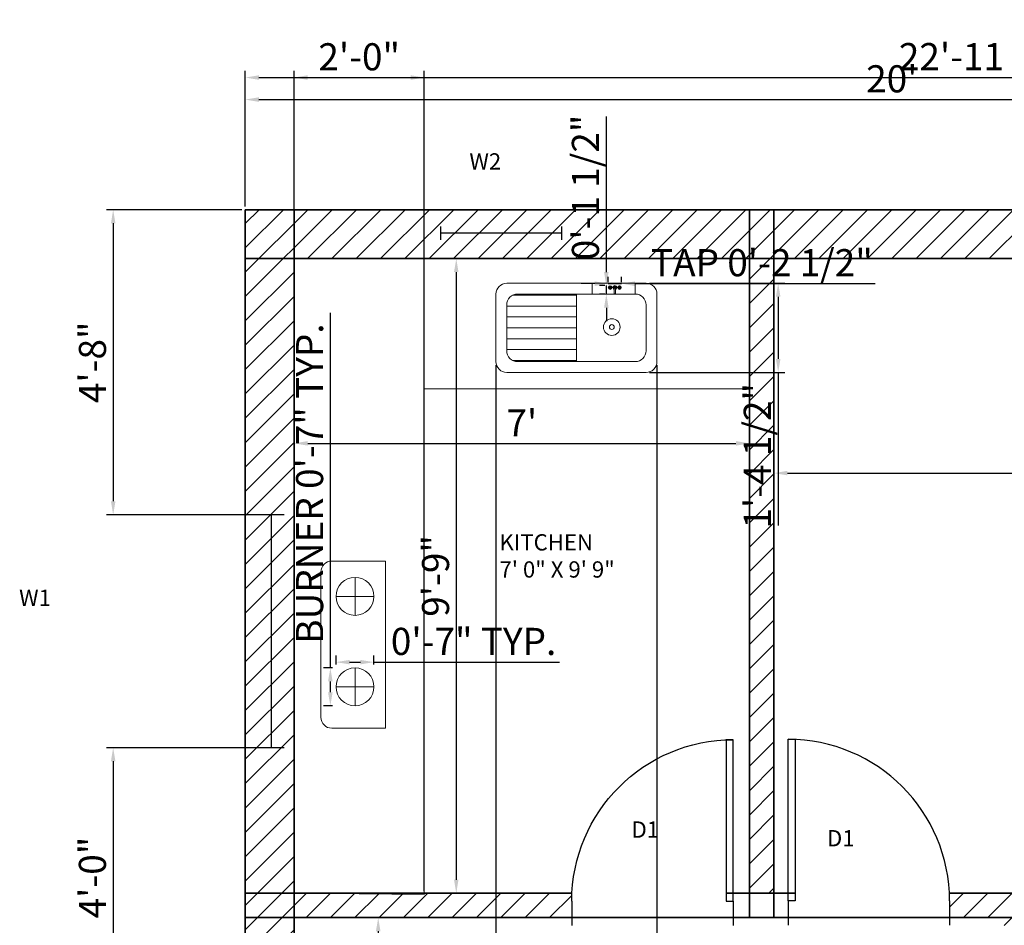
# Model space of a CAD drawing. Units: millimetres. Extents: x 2682 to 3042, y 1647 to 2164.
# Tile 3 of 4: x 2682 to 2864, y 1997 to 2164. Entities that reach past the tile are written whole.
import ezdxf

# ---------------------------------------------------------------- set-up
doc = ezdxf.new("R2010")
doc.units = ezdxf.units.MM
for name, color, linetype, lineweight in [('A-ANNO-TEXT', 170, 'Continuous', 18), ('A-AREA-IDEN', 170, 'Continuous', 18), ('A-EQPM', 220, 'Continuous', 18), ('A-FLOR-CABN', 70, 'Continuous', 18), ('A-FLOR-FIXT', 220, 'Continuous', 18), ('A-WALL-PATT', 3, 'Continuous', 13), ('dimensions', 140, 'Continuous', 18), ('doors', 40, 'Continuous', 25), ('walls', 70, 'Continuous', 35), ('windows', 50, 'Continuous', 25)]:
    doc.layers.add(name, color=color, linetype=linetype, lineweight=lineweight)
doc.styles.get("Standard").update_dxf_attribs({"font": 'arial.ttf'})
doc.dimstyles.new('ISO-25', dxfattribs={"dimtxt": 5, "dimasz": 2.5, "dimexe": 1.25, "dimexo": 0.625, "dimtad": 1, "dimdec": 0, "dimlunit": 3, "dimtxsty": 'Standard', "dimcen": 2.5, "dimadec": 0, "dimazin": 0, "dimtfac": 1, "dimtdec": 0, "dimtmove": 0, "dimatfit": 3, "dimfxl": 1, "dimarcsym": 0})

# ---------------------------------------------------------------- blocks, each defined once
blk = doc.blocks.new('*U2')
for p, q in [((0, 0), (0, -6)), ((40, 0), (40, -6))]:
    blk.add_line(p, q)
blk.add_lwpolyline([(0, 0), (0, 40), (1.75, 40), (1.75, 0)], close=True)
blk.add_arc((0, 0), 40, 0, 90)
blk = doc.blocks.new('*U4')
for p, q in [((0, 4), (0, 0)), ((36, 4), (36, 0)), ((0, 2), (36, 2))]:
    blk.add_line(p, q)
blk = doc.blocks.new('*U5')
for p, q in [((0, 4), (0, 0)), ((36, 4), (36, 0)), ((0, 2), (36, 2))]:
    blk.add_line(p, q)
blk = doc.blocks.new('Faucet - Bathroom top')
for p, q in [((-4.107, 0.125), (-4.375, 0.125)), ((-3.75, 0.4788), (-3.75, 0.75)), ((-3.5, 0.482), (-3.5, 0.75)), ((-3.1461, 0.125), (-2.875, 0.125)), ((3.143, 0.125), (2.875, 0.125)), ((3.5, 0.4788), (3.5, 0.75)), ((3.75, 0.482), (3.75, 0.75)), ((4.1039, 0.125), (4.375, 0.125)), ((-4.1039, -0.125), (-4.375, -0.125)), ((-3.75, -0.4821), (-3.75, -0.75)), ((-3.5, -0.4789), (-3.5, -0.75)), ((-3.143, -0.125), (-2.875, -0.125)), ((-0.5, -0.8639), (-0.5, -4.5)), ((0.5, -4.5), (0.5, -0.8631)), ((3.1461, -0.125), (2.875, -0.125)), ((3.5, -0.4821), (3.5, -0.75)), ((3.75, -0.4789), (3.75, -0.75)), ((4.107, -0.125), (4.375, -0.125))]:
    blk.add_line(p, q)
for centre, radius in [((-3.625, 0), 1.375), ((-4.625, 0), 0.2795), ((-3.625, 0), 0.5), ((-3.625, 1), 0.2795), ((-2.625, 0), 0.2795), ((0, 0), 0.5), ((3.625, 0), 1.375), ((2.625, 0), 0.2795), ((3.625, 0), 0.5), ((3.625, 1), 0.2795), ((4.625, 0), 0.2795), ((-3.625, -1), 0.2795), ((3.625, -1), 0.2795)]:
    blk.add_circle(centre, radius)
for centre, radius, start, end in [((-3.625, 0), 1, 105.2407, 164.2093), ((-3.625, 0), 1, 16.44125, 74.07887), ((0, 0), 1.5, 289.6514, 250.3603), ((0, 0), 1, 300.3431, 239.7554), ((3.625, 0), 1, 106.12, 164.0884), ((3.625, 0), 1, 16.23422, 73.90469), ((-3.625, 0), 1, 196.2342, 253.9047), ((-3.625, 0), 1, 286.12, 344.0884), ((0, -4.5), 0.5, 180, 0), ((3.625, 0), 1, 196.4413, 254.0789), ((3.625, 0), 1, 285.2407, 344.2093)]:
    blk.add_arc(centre, radius, start, end)
blk = doc.blocks.new('*D10')
at = {"layer": 'Defpoints', "color": 0, "transparency": 16777216}
for p in [(2762.5, 2119.93), (2762.5, 2002.93), (2762.5, 2002.93)]:
    blk.add_point(p, dxfattribs=at)
at = {"layer": 'dimensions', "color": 0, "lineweight": -2, "transparency": 16777216}
for p, q in [((2763.12, 2119.93), (2763.75, 2119.93)), ((2762.5, 2117.43), (2762.5, 2005.43)), ((2763.12, 2002.93), (2763.75, 2002.93))]:
    blk.add_line(p, q, dxfattribs=at)
at = {"layer": 'dimensions', "color": 0, "transparency": 16777216}
for points in [[(2762.08, 2117.43), (2762.91, 2117.43), (2762.5, 2119.93)], [(2762.08, 2005.43), (2762.91, 2005.43), (2762.5, 2002.93)]]:
    blk.add_solid(points, dxfattribs=at)
at = {"layer": 'dimensions', "color": 0, "transparency": 16777216, "insert": (2759.32, 2061.43), "char_height": 5, "attachment_point": 5, "rotation": 90}
blk.add_mtext('9\'-9"', dxfattribs=at)
blk = doc.blocks.new('*D11')
at = {"layer": 'Defpoints', "color": 0, "transparency": 16777216}
for p in [(2816.59, 2085.86), (2732.59, 2082.58), (2816.59, 2082.58)]:
    blk.add_point(p, dxfattribs=at)
at = {"layer": 'dimensions', "color": 0, "lineweight": -2, "transparency": 16777216}
for p, q in [((2732.59, 2083.21), (2732.59, 2087.11)), ((2816.59, 2083.21), (2816.59, 2087.11)), ((2735.09, 2085.86), (2814.09, 2085.86))]:
    blk.add_line(p, q, dxfattribs=at)
at = {"layer": 'dimensions', "color": 0, "transparency": 16777216}
for points in [[(2735.09, 2086.28), (2735.09, 2085.45), (2732.59, 2085.86)], [(2814.09, 2086.28), (2814.09, 2085.45), (2816.59, 2085.86)]]:
    blk.add_solid(points, dxfattribs=at)
at = {"layer": 'dimensions', "color": 0, "transparency": 16777216, "insert": (2774.59, 2088.99), "char_height": 5, "attachment_point": 5}
blk.add_mtext("7'", dxfattribs=at)
blk = doc.blocks.new('*D12')
at = {"layer": 'Defpoints', "color": 0, "transparency": 16777216}
for p in [(2821.09, 2090.07), (2953.09, 2090.07), (2953.09, 2080.38)]:
    blk.add_point(p, dxfattribs=at)
at = {"layer": 'dimensions', "color": 0, "lineweight": -2, "transparency": 16777216}
for p, q in [((2821.09, 2089.45), (2821.09, 2079.13)), ((2953.09, 2089.45), (2953.09, 2079.13)), ((2823.59, 2080.38), (2950.59, 2080.38))]:
    blk.add_line(p, q, dxfattribs=at)
at = {"layer": 'dimensions', "color": 0, "transparency": 16777216}
for points in [[(2823.59, 2080.8), (2823.59, 2079.97), (2821.09, 2080.38)], [(2950.59, 2080.8), (2950.59, 2079.97), (2953.09, 2080.38)]]:
    blk.add_solid(points, dxfattribs=at)
at = {"layer": 'dimensions', "color": 0, "transparency": 16777216, "insert": (2887.09, 2083.52), "char_height": 5, "attachment_point": 5}
blk.add_mtext("11'", dxfattribs=at)
blk = doc.blocks.new('*D25')
at = {"layer": 'Defpoints', "color": 0, "transparency": 16777216}
for p in [(2751.08, 1998.43), (2748.1, 1809.43), (2751.08, 1809.43)]:
    blk.add_point(p, dxfattribs=at)
at = {"layer": 'dimensions', "color": 0, "lineweight": -2, "transparency": 16777216}
for p, q in [((2750.46, 1998.43), (2746.85, 1998.43)), ((2748.1, 1995.93), (2748.1, 1811.93)), ((2750.46, 1809.43), (2746.85, 1809.43))]:
    blk.add_line(p, q, dxfattribs=at)
at = {"layer": 'dimensions', "color": 0, "transparency": 16777216}
for points in [[(2747.68, 1995.93), (2748.52, 1995.93), (2748.1, 1998.43)], [(2747.68, 1811.93), (2748.52, 1811.93), (2748.1, 1809.43)]]:
    blk.add_solid(points, dxfattribs=at)
at = {"layer": 'dimensions', "color": 0, "transparency": 16777216, "insert": (2744.92, 1903.93), "char_height": 5, "attachment_point": 5, "rotation": 90}
blk.add_mtext('15\'-9"', dxfattribs=at)
blk = doc.blocks.new('*D28')
at = {"layer": 'Defpoints', "color": 0, "transparency": 16777216}
for p in [(2962.09, 2149.24), (2723.59, 2128.93), (2962.09, 2128.93)]:
    blk.add_point(p, dxfattribs=at)
at = {"layer": 'dimensions', "color": 0, "lineweight": -2, "transparency": 16777216}
for p, q in [((2723.59, 2129.55), (2723.59, 2150.49)), ((2962.09, 2129.55), (2962.09, 2150.49)), ((2726.09, 2149.24), (2959.59, 2149.24))]:
    blk.add_line(p, q, dxfattribs=at)
at = {"layer": 'dimensions', "color": 0, "transparency": 16777216}
for points in [[(2726.09, 2149.66), (2726.09, 2148.82), (2723.59, 2149.24)], [(2959.59, 2149.66), (2959.59, 2148.82), (2962.09, 2149.24)]]:
    blk.add_solid(points, dxfattribs=at)
at = {"layer": 'dimensions', "color": 0, "transparency": 16777216, "insert": (2842.84, 2152.42), "char_height": 5, "width": 20.59, "attachment_point": 5}
blk.add_mtext("20'", dxfattribs=at)
blk = doc.blocks.new('COOKTOP-BURNER')
for p, q in [((3.5, 7), (3.5, 0)), ((3.5, 3.5), (0, 3.5)), ((0, 3.5), (7, 3.5))]:
    blk.add_line(p, q)
blk.add_circle((3.5, 3.5), 3.5)
blk = doc.blocks.new('*D43')
at = {"layer": 'Defpoints', "color": 0, "transparency": 16777216}
for p in [(2739.27, 2044.48), (2740.32, 2044.48), (2740.32, 2037.48)]:
    blk.add_point(p, dxfattribs=at)
at = {"layer": 'dimensions', "color": 0, "lineweight": -2, "transparency": 16777216}
for p, q in [((2739.27, 2044.48), (2739.27, 2109.92)), ((2739.69, 2044.48), (2738.02, 2044.48)), ((2739.27, 2039.98), (2739.27, 2041.98)), ((2739.69, 2037.48), (2738.02, 2037.48))]:
    blk.add_line(p, q, dxfattribs=at)
at = {"layer": 'dimensions', "color": 0, "transparency": 16777216}
for points in [[(2738.85, 2041.98), (2739.69, 2041.98), (2739.27, 2044.48)], [(2738.85, 2039.98), (2739.69, 2039.98), (2739.27, 2037.48)]]:
    blk.add_solid(points, dxfattribs=at)
at = {"layer": 'dimensions', "color": 0, "transparency": 16777216, "insert": (2736.09, 2078.45), "char_height": 5, "attachment_point": 5, "rotation": 90}
blk.add_mtext('BURNER 0\'-7" TYP.', dxfattribs=at)
blk = doc.blocks.new('*D44')
at = {"layer": 'Defpoints', "color": 0, "transparency": 16777216}
for p in [(2747.32, 2045.53), (2740.32, 2044.48), (2747.32, 2044.48)]:
    blk.add_point(p, dxfattribs=at)
at = {"layer": 'dimensions', "color": 0, "lineweight": -2, "transparency": 16777216}
for p, q in [((2740.32, 2045.11), (2740.32, 2046.78)), ((2742.82, 2045.53), (2744.82, 2045.53)), ((2747.32, 2045.11), (2747.32, 2046.78)), ((2747.32, 2045.53), (2781.55, 2045.53))]:
    blk.add_line(p, q, dxfattribs=at)
at = {"layer": 'dimensions', "color": 0, "transparency": 16777216}
for points in [[(2742.82, 2045.95), (2742.82, 2045.12), (2740.32, 2045.53)], [(2744.82, 2045.95), (2744.82, 2045.12), (2747.32, 2045.53)]]:
    blk.add_solid(points, dxfattribs=at)
at = {"layer": 'dimensions', "color": 0, "transparency": 16777216, "insert": (2765.69, 2048.71), "char_height": 5, "attachment_point": 5}
blk.add_mtext('0\'-7" TYP.', dxfattribs=at)
blk = doc.blocks.new('*D45')
at = {"layer": 'Defpoints', "color": 0, "transparency": 16777216}
for p in [(2790.54, 2114.94), (2792.95, 2115.31), (2792.95, 2114.94)]:
    blk.add_point(p, dxfattribs=at)
at = {"layer": 'dimensions', "color": 0, "lineweight": -2, "transparency": 16777216}
for p, q in [((2790.54, 2115.57), (2790.54, 2116.56)), ((2792.95, 2115.57), (2792.95, 2116.56)), ((2788.04, 2115.31), (2785.54, 2115.31)), ((2790.54, 2115.31), (2792.95, 2115.31)), ((2795.45, 2115.31), (2839.79, 2115.31))]:
    blk.add_line(p, q, dxfattribs=at)
at = {"layer": 'dimensions', "color": 0, "transparency": 16777216}
for points in [[(2788.04, 2115.72), (2788.04, 2114.89), (2790.54, 2115.31)], [(2795.45, 2115.72), (2795.45, 2114.89), (2792.95, 2115.31)]]:
    blk.add_solid(points, dxfattribs=at)
at = {"layer": 'dimensions', "color": 0, "transparency": 16777216, "insert": (2818.87, 2118.52), "char_height": 5, "attachment_point": 5}
blk.add_mtext('TAP 0\'-2 1/2"', dxfattribs=at)
blk = doc.blocks.new('*D46')
at = {"layer": 'Defpoints', "color": 0, "transparency": 16777216}
for p in [(2790.18, 2114.94), (2790.54, 2114.94), (2790.54, 2113.38)]:
    blk.add_point(p, dxfattribs=at)
at = {"layer": 'dimensions', "color": 0, "lineweight": -2, "transparency": 16777216}
for p, q in [((2790.18, 2117.44), (2790.18, 2146.14)), ((2789.92, 2114.94), (2788.93, 2114.94)), ((2790.18, 2113.38), (2790.18, 2114.94)), ((2789.92, 2113.38), (2788.93, 2113.38)), ((2790.18, 2110.88), (2790.18, 2108.38))]:
    blk.add_line(p, q, dxfattribs=at)
at = {"layer": 'dimensions', "color": 0, "transparency": 16777216}
for points in [[(2789.76, 2117.44), (2790.6, 2117.44), (2790.18, 2114.94)], [(2789.76, 2110.88), (2790.6, 2110.88), (2790.18, 2113.38)]]:
    blk.add_solid(points, dxfattribs=at)
at = {"layer": 'dimensions', "color": 0, "transparency": 16777216, "insert": (2786.97, 2133.04), "char_height": 5, "attachment_point": 5, "rotation": 90}
blk.add_mtext('0\'-1 1/2"', dxfattribs=at)
blk = doc.blocks.new('*D51')
at = {"layer": 'Defpoints', "color": 0, "transparency": 16777216}
for p in [(2797.51, 2115.38), (2797.51, 2098.93), (2821.88, 2098.93)]:
    blk.add_point(p, dxfattribs=at)
at = {"layer": 'dimensions', "color": 0, "lineweight": -2, "transparency": 16777216}
for p, q in [((2798.13, 2115.38), (2823.13, 2115.38)), ((2821.88, 2112.88), (2821.88, 2101.43)), ((2798.13, 2098.93), (2823.13, 2098.93)), ((2821.88, 2098.93), (2821.88, 2070.71))]:
    blk.add_line(p, q, dxfattribs=at)
at = {"layer": 'dimensions', "color": 0, "transparency": 16777216}
for points in [[(2821.46, 2112.88), (2822.3, 2112.88), (2821.88, 2115.38)], [(2821.46, 2101.43), (2822.3, 2101.43), (2821.88, 2098.93)]]:
    blk.add_solid(points, dxfattribs=at)
at = {"layer": 'dimensions', "color": 0, "transparency": 16777216, "insert": (2818.67, 2083.57), "char_height": 5, "attachment_point": 5, "rotation": 90}
blk.add_mtext('1\'-4 1/2"', dxfattribs=at)
blk = doc.blocks.new('*D52')
at = {"layer": 'Defpoints', "color": 0, "transparency": 16777216}
for p in [(2769.81, 2100.93), (2799.51, 2100.93), (2799.51, 1651.55)]:
    blk.add_point(p, dxfattribs=at)
at = {"layer": 'dimensions', "color": 0, "lineweight": -2, "transparency": 16777216}
for p, q in [((2769.81, 2100.31), (2769.81, 1650.3)), ((2799.51, 2100.31), (2799.51, 1650.3)), ((2772.31, 1651.55), (2797.01, 1651.55))]:
    blk.add_line(p, q, dxfattribs=at)
at = {"layer": 'dimensions', "color": 0, "transparency": 16777216}
for points in [[(2772.31, 1651.97), (2772.31, 1651.13), (2769.81, 1651.55)], [(2797.01, 1651.97), (2797.01, 1651.13), (2799.51, 1651.55)]]:
    blk.add_solid(points, dxfattribs=at)
at = {"layer": 'dimensions', "color": 0, "transparency": 16777216, "insert": (2784.66, 1654.76), "char_height": 5, "attachment_point": 5}
blk.add_mtext('2\'-5 1/2"', dxfattribs=at)
blk = doc.blocks.new('*D53')
at = {"layer": 'Defpoints', "color": 0, "transparency": 16777216}
for p in [(2999.09, 2153.3), (2723.59, 2128.93), (2999.09, 1950.43)]:
    blk.add_point(p, dxfattribs=at)
at = {"layer": 'dimensions', "color": 0, "lineweight": -2, "transparency": 16777216}
for p, q in [((2723.59, 2129.55), (2723.59, 2154.55)), ((2999.09, 1951.05), (2999.09, 2154.55)), ((2726.09, 2153.3), (2996.59, 2153.3))]:
    blk.add_line(p, q, dxfattribs=at)
at = {"layer": 'dimensions', "color": 0, "transparency": 16777216}
for points in [[(2726.09, 2153.72), (2726.09, 2152.88), (2723.59, 2153.3)], [(2996.59, 2153.72), (2996.59, 2152.88), (2999.09, 2153.3)]]:
    blk.add_solid(points, dxfattribs=at)
at = {"layer": 'dimensions', "color": 0, "transparency": 16777216, "insert": (2861.34, 2156.51), "char_height": 5, "attachment_point": 5}
blk.add_mtext('22\'-11 1/2"', dxfattribs=at)
blk = doc.blocks.new('*D66')
at = {"layer": 'Defpoints', "color": 0, "transparency": 16777216}
for p in [(2756.59, 2153.3), (2732.59, 2002.93), (2756.59, 2002.69)]:
    blk.add_point(p, dxfattribs=at)
at = {"layer": 'dimensions', "color": 0, "lineweight": -2, "transparency": 16777216}
for p, q in [((2732.59, 2003.55), (2732.59, 2154.55)), ((2756.59, 2003.32), (2756.59, 2154.55)), ((2735.09, 2153.3), (2754.09, 2153.3))]:
    blk.add_line(p, q, dxfattribs=at)
at = {"layer": 'dimensions', "color": 0, "transparency": 16777216}
for points in [[(2735.09, 2153.72), (2735.09, 2152.88), (2732.59, 2153.3)], [(2754.09, 2153.72), (2754.09, 2152.88), (2756.59, 2153.3)]]:
    blk.add_solid(points, dxfattribs=at)
at = {"layer": 'dimensions', "color": 0, "transparency": 16777216, "insert": (2744.59, 2156.48), "char_height": 5, "attachment_point": 5}
blk.add_mtext('2\'-0"', dxfattribs=at)
blk = doc.blocks.new('*D67')
at = {"layer": 'Defpoints', "color": 0, "transparency": 16777216}
for p in [(2723.59, 2128.93), (2699.21, 2072.68), (2728.36, 2072.68)]:
    blk.add_point(p, dxfattribs=at)
at = {"layer": 'dimensions', "color": 0, "lineweight": -2, "transparency": 16777216}
for p, q in [((2722.96, 2128.93), (2697.96, 2128.93)), ((2699.21, 2126.43), (2699.21, 2075.18)), ((2727.73, 2072.68), (2697.96, 2072.68))]:
    blk.add_line(p, q, dxfattribs=at)
at = {"layer": 'dimensions', "color": 0, "transparency": 16777216}
for points in [[(2698.8, 2126.43), (2699.63, 2126.43), (2699.21, 2128.93)], [(2698.8, 2075.18), (2699.63, 2075.18), (2699.21, 2072.68)]]:
    blk.add_solid(points, dxfattribs=at)
at = {"layer": 'dimensions', "color": 0, "transparency": 16777216, "insert": (2696.03, 2100.8), "char_height": 5, "attachment_point": 5, "rotation": 90}
blk.add_mtext('4\'-8"', dxfattribs=at)
blk = doc.blocks.new('*D68')
at = {"layer": 'Defpoints', "color": 0, "transparency": 16777216}
for p in [(2728.36, 2029.76), (2699.21, 1981.89), (2728.36, 1981.89)]:
    blk.add_point(p, dxfattribs=at)
at = {"layer": 'dimensions', "color": 0, "lineweight": -2, "transparency": 16777216}
for p, q in [((2727.73, 2029.76), (2697.96, 2029.76)), ((2699.21, 2027.26), (2699.21, 1984.39)), ((2727.73, 1981.89), (2697.96, 1981.89))]:
    blk.add_line(p, q, dxfattribs=at)
at = {"layer": 'dimensions', "color": 0, "transparency": 16777216}
for points in [[(2698.8, 2027.26), (2699.63, 2027.26), (2699.21, 2029.76)], [(2698.8, 1984.39), (2699.63, 1984.39), (2699.21, 1981.89)]]:
    blk.add_solid(points, dxfattribs=at)
at = {"layer": 'dimensions', "color": 0, "transparency": 16777216, "insert": (2696.03, 2005.82), "char_height": 5, "attachment_point": 5, "rotation": 90}
blk.add_mtext('4\'-0"', dxfattribs=at)

msp = doc.modelspace()

# ---------------------------------------------------------------- hatches: boundary and pattern name
at = {"layer": 'A-WALL-PATT'}
h = msp.add_hatch(dxfattribs=at)
h.set_pattern_fill('ANSI31', color=256)
h.paths.add_polyline_path([(2816.59, 2128.93), (2732.59, 2128.93), (2732.59, 2119.93), (2816.59, 2119.93)])
h.paths.add_polyline_path([(2953.09, 2128.93), (2821.09, 2128.93), (2821.09, 2119.93), (2953.09, 2119.93)])
h.paths.add_polyline_path([(2821.09, 2119.93), (2816.59, 2119.93), (2816.59, 2002.93), (2821.09, 2002.93)])
h.paths.add_polyline_path([(2821.09, 2128.93), (2816.59, 2128.93), (2816.59, 2119.93), (2821.09, 2119.93)])
h.paths.add_polyline_path([(2732.59, 2119.93), (2723.59, 2119.93), (2723.59, 2002.93), (2732.59, 2002.93)])
h.paths.add_polyline_path([(2732.59, 2128.93), (2723.59, 2128.93), (2723.59, 2119.93), (2732.59, 2119.93)])
h.paths.add_polyline_path([(2962.09, 2119.93), (2953.09, 2119.93), (2953.09, 2002.93), (2962.09, 2002.93)])
h.paths.add_polyline_path([(2962.09, 2128.93), (2953.09, 2128.93), (2953.09, 2119.93), (2962.09, 2119.93)])
h.paths.add_polyline_path([(2953.09, 2002.93), (2897.45, 2002.93), (2897.45, 2000.43, -0.023466), (2897.35, 1998.43), (2953.09, 1998.43)])
h.paths.add_polyline_path([(2962.09, 1998.43), (2953.09, 1998.43), (2953.09, 1950.43), (2962.09, 1950.43)])
h.paths.add_polyline_path([(2953.09, 1950.43), (2868.09, 1950.43), (2868.09, 1945.93), (2953.09, 1945.93)])
h.paths.add_polyline_path([(2994.59, 1950.43), (2962.09, 1950.43), (2962.09, 1945.93), (2994.59, 1945.93)])
h.paths.add_polyline_path([(2868.09, 1998.43), (2863.59, 1998.43), (2863.59, 1950.43), (2868.09, 1950.43)])
h.paths.add_polyline_path([(2868.09, 2002.93), (2863.59, 2002.93), (2863.59, 1998.43), (2868.09, 1998.43)])
h.paths.add_polyline_path([(2863.59, 2002.93), (2853.46, 2002.93, -0.011786), (2853.49, 2001.52), (2853.49, 1998.43), (2863.59, 1998.43)])
h.paths.add_polyline_path([(2783.8, 2001.45, -0.012351), (2783.84, 2002.93), (2756.59, 2002.93), (2756.59, 2002.69), (2732.59, 2002.93), (2732.59, 1998.43), (2783.8, 1998.43)])
h.paths.add_polyline_path([(2732.59, 2002.93), (2723.59, 2002.93), (2723.59, 1998.43), (2732.59, 1998.43)])
h.paths.add_polyline_path([(2732.59, 1998.43), (2723.59, 1998.43), (2723.59, 1809.43), (2732.59, 1809.43)])
h.paths.add_polyline_path([(2994.59, 1861.93), (2962.09, 1861.93), (2962.09, 1857.43), (2994.59, 1857.43)])
h.paths.add_polyline_path([(2999.09, 1884.37), (2994.59, 1884.37), (2994.59, 1861.93), (2999.09, 1861.93)])
h.paths.add_polyline_path([(2953.09, 1861.93), (2868.09, 1861.93), (2868.09, 1857.43), (2953.09, 1857.43)])
h.paths.add_polyline_path([(2962.09, 1861.93), (2953.09, 1861.93), (2953.09, 1857.43), (2962.09, 1857.43)])
h.paths.add_polyline_path([(2868.09, 1857.43), (2863.59, 1857.43), (2863.59, 1831.73), (2866.39, 1831.73, -0.019816), (2868.09, 1831.66)])
h.paths.add_polyline_path([(2868.09, 1861.93), (2863.59, 1861.93), (2863.59, 1857.43), (2868.09, 1857.43)])
h.paths.add_polyline_path([(2962.09, 1804.93), (2953.09, 1804.93), (2953.09, 1684.93), (2962.09, 1684.93)])
h.paths.add_polyline_path([(2962.09, 1857.43), (2953.09, 1857.43), (2953.09, 1809.43), (2962.09, 1809.43)])
h.paths.add_polyline_path([(2962.09, 1809.43), (2953.09, 1809.43), (2953.09, 1804.93), (2962.09, 1804.93)])
h.paths.add_polyline_path([(2953.09, 1809.43), (2868.09, 1809.43), (2868.09, 1804.93), (2953.09, 1804.93)])
h.paths.add_polyline_path([(2868.09, 1809.43), (2863.59, 1809.43), (2863.59, 1804.93), (2868.09, 1804.93)])
h.paths.add_polyline_path([(2863.59, 1809.43), (2855.42, 1809.43), (2855.42, 1805.73, -0.006742), (2855.41, 1804.93), (2863.59, 1804.93)])
h.paths.add_polyline_path([(2953.09, 1684.93), (2863.59, 1684.93), (2821.09, 1684.93), (2821.09, 1675.93), (2863.59, 1675.93), (2953.09, 1675.93)])
h.paths.add_polyline_path([(2962.09, 1684.93), (2953.09, 1684.93), (2953.09, 1675.93), (2962.09, 1675.93)])
h.paths.add_polyline_path([(2821.09, 1804.93), (2816.59, 1804.93), (2816.59, 1704.93), (2821.09, 1704.93)])
h.paths.add_polyline_path([(2821.09, 1695.93), (2816.59, 1695.93), (2816.59, 1684.93), (2821.09, 1684.93)])
h.paths.add_polyline_path([(2821.09, 1704.93), (2816.59, 1704.93), (2816.59, 1695.93), (2821.09, 1695.93)])
h.paths.add_polyline_path([(2821.09, 1684.93), (2816.59, 1684.93), (2816.59, 1675.93), (2821.09, 1675.93)])
h.paths.add_polyline_path([(2776.38, 1700.56, -0.030957), (2776.65, 1704.93), (2732.59, 1704.93), (2732.59, 1695.93), (2776.38, 1695.93)])
h.paths.add_polyline_path([(2732.59, 1804.93), (2723.59, 1804.93), (2723.59, 1704.93), (2732.59, 1704.93)])
h.paths.add_polyline_path([(2732.59, 1704.93), (2723.59, 1704.93), (2723.59, 1695.93), (2732.59, 1695.93)])
h.paths.add_polyline_path([(2999.09, 1945.93), (2994.59, 1945.93), (2994.59, 1937.59), (2999.09, 1937.59)])
h.paths.add_polyline_path([(2999.09, 1937.59), (2996.77, 1937.59), (2996.77, 1884.37), (2999.09, 1884.37)])
h.paths.add_polyline_path([(2996.77, 1937.59), (2994.59, 1937.59), (2994.59, 1884.37), (2996.77, 1884.37)])
h.paths.add_polyline_path([(2784.83, 1809.43), (2732.59, 1809.43), (2732.59, 1804.93), (2784.84, 1804.93, -0.006742), (2784.83, 1805.73)])
h.paths.add_polyline_path([(2732.59, 1809.43), (2723.59, 1809.43), (2723.59, 1804.93), (2732.59, 1804.93)])

# ---------------------------------------------------------------- linework, layer by layer
at = {"layer": 'A-EQPM'}
msp.add_lwpolyline([(2739.52, 2064.16), (2749.42, 2064.16), (2749.42, 2033.36), (2739.52, 2033.36, -0.414214), (2737.52, 2035.36), (2737.52, 2062.16, -0.414214)], format="xyb", close=True, dxfattribs=at)
at = {"layer": 'A-FLOR-CABN'}
for p, q in [((2756.59, 2002.69), (2756.59, 2095.93)), ((2756.59, 2095.93), (2816.59, 2095.93)), ((2732.59, 2002.93), (2756.59, 2002.69))]:
    msp.add_line(p, q, dxfattribs=at)
at = {"layer": 'A-FLOR-FIXT'}
for p, q in [((2772.89, 2113.16), (2784.66, 2113.16)), ((2784.66, 2113.38), (2784.66, 2100.93)), ((2771.81, 2111.16), (2784.66, 2111.16)), ((2771.81, 2109.16), (2784.66, 2109.16)), ((2771.81, 2107.16), (2784.66, 2107.16)), ((2771.81, 2105.16), (2784.66, 2105.16)), ((2771.81, 2103.16), (2784.66, 2103.16)), ((2772.89, 2101.16), (2784.66, 2101.16))]:
    msp.add_line(p, q, dxfattribs=at)
for points in [[(2771.81, 2115.38), (2797.51, 2115.38, -0.414214), (2799.51, 2113.38), (2799.51, 2100.93, -0.414214), (2797.51, 2098.93), (2771.81, 2098.93, -0.414214), (2769.81, 2100.93), (2769.81, 2113.38, -0.414214)], [(2773.81, 2113.38), (2795.51, 2113.38, -0.414214), (2797.51, 2111.38), (2797.51, 2102.93, -0.414214), (2795.51, 2100.93), (2773.81, 2100.93, -0.414214), (2771.81, 2102.93), (2771.81, 2111.38, -0.414214)]]:
    msp.add_lwpolyline(points, format="xyb", close=True, dxfattribs=at)
msp.add_lwpolyline([(2787.57, 2115.38), (2795.51, 2115.38), (2795.51, 2113.38), (2787.57, 2113.38)], close=True, dxfattribs=at)
for radius in [1.54, 0.439]:
    msp.add_circle((2791.19, 2107.31), radius, dxfattribs=at)
at = {"layer": 'walls'}
for p, q in [((2723.59, 2128.93), (2723.59, 1695.93)), ((2723.59, 2128.93), (2962.09, 2128.93)), ((2732.59, 2128.93), (2732.59, 1695.93)), ((2816.59, 2128.93), (2816.59, 1998.43)), ((2821.09, 2128.93), (2821.09, 1998.43)), ((2723.59, 2119.93), (2962.09, 2119.93)), ((2723.59, 2002.93), (2783.84, 2002.93)), ((2812.29, 2002.93), (2825.01, 2002.93)), ((2853.46, 2002.93), (2962.09, 2002.93)), ((2723.59, 1998.43), (2876.97, 1998.43))]:
    msp.add_line(p, q, dxfattribs=at)

# ---------------------------------------------------------------- block references
at = {"layer": 'A-EQPM', "rotation": 180}
msp.add_blockref('COOKTOP-BURNER', (2747.32, 2061.16), dxfattribs=at)
at = {"layer": 'A-EQPM'}
msp.add_blockref('COOKTOP-BURNER', (2740.32, 2037.48), dxfattribs=at)
at = {"layer": 'A-FLOR-FIXT', "xscale": 0.2405482146988106, "yscale": 0.2405482146988106, "zscale": 0.2405482146988106}
msp.add_blockref('Faucet - Bathroom top', (2791.74, 2114.58), dxfattribs=at)
at = {"layer": 'doors', "yscale": 0.744697270728857, "zscale": 0.744697270728857}
for p, xscale in [((2813.59, 2001.45), -0.744697270728857), ((2823.7, 2001.52), 0.744697270728857)]:
    msp.add_blockref('*U2', p, dxfattribs=dict(at, xscale=xscale))
at = {"layer": 'windows'}
for name, p, xscale, yscale, zscale, rotation in [('*U5', (2781.99, 2125.85), 0.6208711624712905, 0.6208711624712905, 0.6208711624712905, 180), ('*U4', (2725.97, 2072.68), 1.192221816707046, 1.192221816707046, 1.192221816707046, 270)]:
    msp.add_blockref(name, p, dxfattribs=dict(at, xscale=xscale, yscale=yscale, zscale=zscale, rotation=rotation))

# ---------------------------------------------------------------- texts
at = {"layer": 'A-ANNO-TEXT', "char_height": 3, "attachment_point": 1}
for s, width, insert in [('W2', 13.9941, (2764.92, 2139.34)), ('W1', 30.2219, (2681.86, 2058.89)), ('D1', 9.5418, (2794.83, 2016.17)), ('D1', 16.3298, (2830.88, 2014.57))]:
    msp.add_mtext_dynamic_manual_height_columns(s, width=width, gutter_width=12.5, heights=[0], dxfattribs=dict(at, insert=insert))
at = {"layer": 'A-AREA-IDEN', "insert": (2770.47, 2069.12), "char_height": 3, "attachment_point": 1}
msp.add_mtext_dynamic_manual_height_columns('KITCHEN\\P7\' 0" X 9\' 9"', width=29.9047, gutter_width=12.5, heights=[0], dxfattribs=at)

# ---------------------------------------------------------------- dimensions: what is measured, and where the dimension line sits
at = {"layer": 'dimensions'}
for base, p1, p2, override, picture, middle in [((2999.09, 2153.3), (2723.59, 2128.93), (2999.09, 1950.43), {"dimdec": 1, "dimlfac": 1, "dimrnd": 0, "dimzin": 1, "dimdsep": 46, "dimlunit": 4, "dimfrac": 2}, '*D53', (2861.34, 2156.51)), ((2756.59, 2153.3), (2732.59, 2002.93), (2756.59, 2002.69), {"dimdec": 1, "dimlfac": 1, "dimrnd": 0, "dimzin": 1, "dimdsep": 46, "dimlunit": 4, "dimfrac": 2}, '*D66', (2744.59, 2156.48)), ((2799.51, 1651.55), (2769.81, 2100.93), (2799.51, 2100.93), {"dimdec": 1, "dimlfac": 1, "dimrnd": 0, "dimzin": 1, "dimdsep": 46, "dimlunit": 4, "dimfrac": 2}, '*D52', (2784.66, 1654.76)), ((2816.59, 2085.86), (2732.59, 2082.58), (2816.59, 2082.58), {"dimclrd": 0, "dimclre": 0, "dimclrt": 0}, '*D11', (2774.59, 2088.99)), ((2953.09, 2080.38), (2821.09, 2090.07), (2953.09, 2090.07), {"dimclrd": 0, "dimclre": 0, "dimclrt": 0}, '*D12', (2887.09, 2083.52))]:
    dim = msp.add_linear_dim(base=base, p1=p1, p2=p2, dimstyle='ISO-25', override=override, dxfattribs=at)
    dim.commit()
    dim.dimension.update_dxf_attribs({"geometry": picture, "text_midpoint": middle})
for base, p1, p2, text, override, picture, middle in [((2962.09, 2149.24), (2723.59, 2128.93), (2962.09, 2128.93), "20'", {"dimclrd": 0, "dimclre": 0, "dimclrt": 0}, '*D28', (2842.84, 2152.42)), ((2792.95, 2115.31), (2790.54, 2114.94), (2792.95, 2114.94), 'TAP <>', {"dimdec": 1, "dimlfac": 1, "dimrnd": 0, "dimzin": 1, "dimdsep": 46, "dimlunit": 4, "dimfrac": 2}, '*D45', (2818.87, 2118.52)), ((2747.32, 2045.53), (2740.32, 2044.48), (2747.32, 2044.48), '<> TYP.', {"dimdec": 1, "dimlfac": 1, "dimrnd": 0, "dimzin": 1, "dimdsep": 46, "dimlunit": 4, "dimfrac": 2}, '*D44', (2765.69, 2048.71))]:
    dim = msp.add_linear_dim(base=base, p1=p1, p2=p2, text=text, dimstyle='ISO-25', override=override, dxfattribs=at)
    dim.commit()
    dim.dimension.update_dxf_attribs({"geometry": picture, "text_midpoint": middle})
for base, p1, p2, angle, override, picture, middle in [((2790.18, 2114.94), (2790.54, 2113.38), (2790.54, 2114.94), 90, {"dimdec": 1, "dimlfac": 1, "dimrnd": 0, "dimzin": 1, "dimdsep": 46, "dimlunit": 4, "dimfrac": 2}, '*D46', (2786.97, 2133.04)), ((2699.2122, 2072.67533), (2723.5872, 2128.92528), (2728.35608, 2072.67533), 90, {"dimdec": 1, "dimlfac": 1, "dimrnd": 0, "dimzin": 1, "dimdsep": 46, "dimlunit": 4, "dimfrac": 2}, '*D67', (2696.03433, 2100.80031)), ((2762.5, 2002.93), (2762.5, 2119.93), (2762.5, 2002.93), 90, {"dimclrd": 0, "dimclre": 0, "dimclrt": 0}, '*D10', (2759.32, 2061.43)), ((2821.8804, 2098.9316), (2797.5054, 2115.3805), (2797.5054, 2098.9316), 270, {"dimdec": 1, "dimlfac": 1, "dimrnd": 0, "dimzin": 1, "dimdsep": 46, "dimlunit": 4, "dimfrac": 2}, '*D51', (2818.6701, 2083.5709)), ((2699.21, 1981.89), (2728.36, 2029.76), (2728.36, 1981.89), 90, {"dimdec": 1, "dimlfac": 1, "dimrnd": 0, "dimzin": 1, "dimdsep": 46, "dimlunit": 4, "dimfrac": 2}, '*D68', (2696.03, 2005.82)), ((2748.1, 1809.43), (2751.08, 1998.43), (2751.08, 1809.43), 90, {"dimclrd": 0, "dimclre": 0, "dimclrt": 0}, '*D25', (2744.92, 1903.93))]:
    dim = msp.add_linear_dim(base=base, p1=p1, p2=p2, angle=angle, dimstyle='ISO-25', override=override, dxfattribs=at)
    dim.commit()
    dim.dimension.update_dxf_attribs({"geometry": picture, "text_midpoint": middle})
dim = msp.add_linear_dim(base=(2739.27, 2044.48), p1=(2740.32, 2037.48), p2=(2740.32, 2044.48), angle=90, text='BURNER <> TYP.', dimstyle='ISO-25', override={"dimdec": 1, "dimlfac": 1, "dimrnd": 0, "dimzin": 1, "dimdsep": 46, "dimlunit": 4, "dimfrac": 2}, dxfattribs=at)
dim.commit()
dim.dimension.update_dxf_attribs({"geometry": '*D43', "text_midpoint": (2736.09, 2078.45)})

doc.saveas('drawing.dxf')
